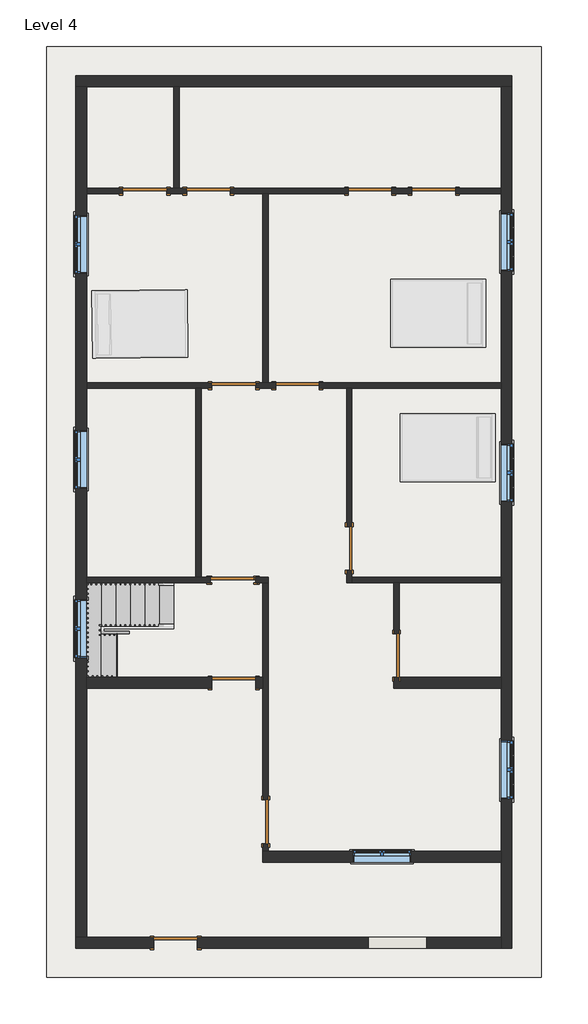
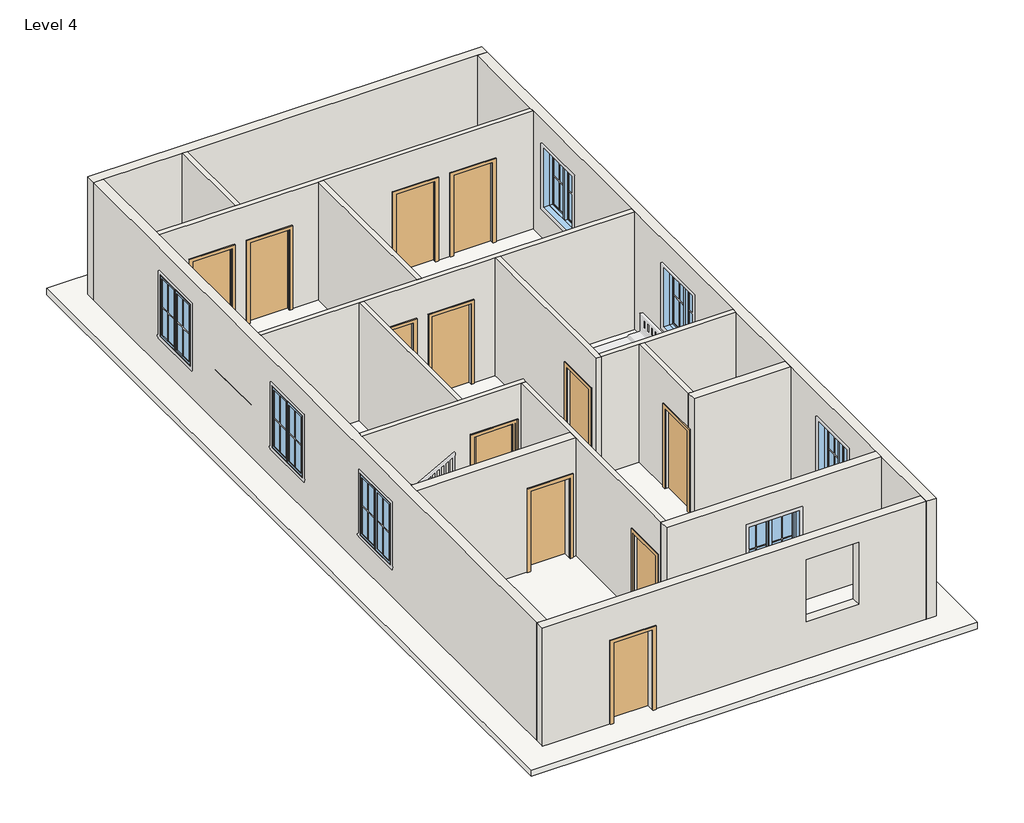
# One storey, part 1 of 2: 17 walls, 13 doors, 7 windows, 1 roof, 1 stair flight.
"""IFC4 building model written with IfcOpenShell, lengths in millimetres."""

from ifc_helpers import new_model, si_unit, frame, origin, place, context, project, spatial, polyline, outline, extrude, faceted_brep, transform, mapped, element, save
from components import door_e5f9f3c4, door_305aa2a5, door_0ca8825f, stair_flight_f33635a8, window_8377141f

model = new_model("IFC4")

# Units and contexts
model_context = context("Model", 3, world=origin())
ifc_project = project(units=[si_unit("LENGTHUNIT", "METRE", prefix="MILLI")], contexts=[model_context])

# Site, building, storey
site = spatial("IfcSite", under=ifc_project)
building = spatial("IfcBuilding", under=site)
storey = spatial("IfcBuildingStorey", under=building, Name="Level 4", Elevation=9144.0)

# Doors
placement = place(None, origin())
door_shape = door_e5f9f3c4(model_context)
element("IfcDoor", 1, ObjectType="Single-Flush : 36\" x 84\"", at=placement, inside=storey, context=model_context, shape_type="MappedRepresentation", body=[
    mapped(door_shape, transform((7442.2, 11550.65, 9144.0), x_axis=(1.0, 0.0, 0.0), y_axis=(0.0, 1.0, 0.0), z_axis=(0.0, 0.0, 1.0))),
])
element("IfcDoor", 2, ObjectType="Single-Flush : 36\" x 84\"", at=placement, inside=storey, context=model_context, shape_type="MappedRepresentation", body=[
    mapped(door_shape, transform((2717.8, 11550.65, 9144.0), x_axis=(1.0, 0.0, 0.0), y_axis=(0.0, 1.0, 0.0), z_axis=(0.0, 0.0, 1.0))),
])
element("IfcDoor", 3, ObjectType="Single-Flush : 36\" x 84\"", at=placement, inside=storey, context=model_context, shape_type="MappedRepresentation", body=[
    mapped(door_shape, transform((4584.7, 7473.95, 9144.0), x_axis=(1.0, 0.0, 0.0), y_axis=(0.0, 1.0, 0.0), z_axis=(0.0, 0.0, 1.0))),
])
element("IfcDoor", 4, ObjectType="Single-Flush : 36\" x 84\"", at=placement, inside=storey, context=model_context, shape_type="MappedRepresentation", body=[
    mapped(door_shape, transform((4546.6, 3397.25, 9144.0), x_axis=(1.0, 0.0, 0.0), y_axis=(0.0, 1.0, 0.0), z_axis=(0.0, 0.0, 1.0))),
])
element("IfcDoor", 5, ObjectType="Single-Flush : 36\" x 84\"", at=placement, inside=storey, context=model_context, shape_type="MappedRepresentation", body=[
    mapped(door_shape, transform((4584.7, 3397.25, 9144.0), x_axis=(1.0, 0.0, 0.0), y_axis=(0.0, 1.0, 0.0), z_axis=(0.0, 0.0, 1.0))),
])
element("IfcDoor", 6, ObjectType="Single-Flush : 36\" x 84\"", at=placement, inside=storey, context=model_context, shape_type="MappedRepresentation", body=[
    mapped(door_shape, transform((7004.05, 4064.0, 9144.0), x_axis=(0.0, -1.0, 0.0), y_axis=(1.0, 0.0, 0.0), z_axis=(0.0, 0.0, 1.0))),
])
element("IfcDoor", 7, ObjectType="Single-Flush : 36\" x 84\"", at=placement, inside=storey, context=model_context, shape_type="MappedRepresentation", body=[
    mapped(door_shape, transform((5251.45, -1663.7, 9144.0), x_axis=(0.0, -1.0, 0.0), y_axis=(1.0, 0.0, 0.0), z_axis=(0.0, 0.0, 1.0))),
])
door_2_shape = door_305aa2a5(model_context)
element("IfcDoor", 8, ObjectType="Single-Flush : 36\" x 84\"", at=placement, inside=storey, context=model_context, shape_type="MappedRepresentation", body=[
    mapped(door_2_shape, transform((4051.3, 11550.65, 9144.0), x_axis=(-1.0, 0.0, 0.0), y_axis=(0.0, -1.0, 0.0), z_axis=(0.0, 0.0, 1.0))),
])
element("IfcDoor", 9, ObjectType="Single-Flush : 36\" x 84\"", at=placement, inside=storey, context=model_context, shape_type="MappedRepresentation", body=[
    mapped(door_2_shape, transform((5918.2, 7473.95, 9144.0), x_axis=(-1.0, 0.0, 0.0), y_axis=(0.0, -1.0, 0.0), z_axis=(0.0, 0.0, 1.0))),
])
element("IfcDoor", 10, ObjectType="Single-Flush : 36\" x 84\"", at=placement, inside=storey, context=model_context, shape_type="MappedRepresentation", body=[
    mapped(door_2_shape, transform((7994.65, 1816.1, 9144.0), x_axis=(0.0, 1.0, 0.0), y_axis=(-1.0, 0.0, 0.0), z_axis=(0.0, 0.0, 1.0))),
])
element("IfcDoor", 11, ObjectType="Single-Flush : 36\" x 84\"", at=placement, inside=storey, context=model_context, shape_type="MappedRepresentation", body=[
    mapped(door_2_shape, transform((8775.7, 11550.65, 9144.0), x_axis=(-1.0, 0.0, 0.0), y_axis=(0.0, -1.0, 0.0), z_axis=(0.0, 0.0, 1.0))),
])
door_3_shape = door_0ca8825f(model_context)
element("IfcDoor", 12, ObjectType="Single-Flush : 36\" x 84\"", at=placement, inside=storey, context=model_context, shape_type="MappedRepresentation", body=[
    mapped(door_3_shape, transform((4584.7, 1244.6, 9144.0), x_axis=(1.0, 0.0, 0.0), y_axis=(0.0, 1.0, 0.0), z_axis=(0.0, 0.0, 1.0))),
])
element("IfcDoor", 13, ObjectType="Single-Flush : 36\" x 84\"", at=placement, inside=storey, context=model_context, shape_type="MappedRepresentation", body=[
    mapped(door_3_shape, transform((3365.5, -4203.7, 9144.0), x_axis=(1.0, 0.0, 0.0), y_axis=(0.0, 1.0, 0.0), z_axis=(0.0, 0.0, 1.0))),
])

# Roof
element("IfcRoof", 14, ObjectType="Generic - 12\"", at=placement, inside=storey, context=model_context, shape_type="SweptSolid", body=[
    extrude(outline(polyline([(660.4, 14579.6), (11023.6, 14579.6), (11023.6, -4927.6), (660.4, -4927.6), (660.4, 14579.6)])), frame((0.0, 0.0, 9144.0), z_axis=(0.0, 0.0, 1.0), x_axis=(1.0, 0.0, 0.0)), (0.0, 0.0, 1.0), 152.4),
])

# Stair flight
stair_flight_shape = stair_flight_f33635a8(model_context)
element("IfcStairFlight", 15, ObjectType="2\" Tread 1\" Nosing 1/4\" Riser", at=placement, inside=storey, context=model_context, shape_type="MappedRepresentation", body=[
    mapped(stair_flight_shape, transform((0.0, 0.0, 0.0), x_axis=(1.0, 0.0, 0.0), y_axis=(0.0, 1.0, 0.0), z_axis=(0.0, 0.0, 1.0))),
])

# Walls
element("IfcWall", 16, ObjectType="Generic - 5\"", at=placement, inside=storey, context=model_context, shape_type="SweptSolid", body=[
    extrude(outline(polyline([(3327.4, 11607.8), (3327.4, 13741.4), (3441.7, 13741.4), (3441.7, 11607.8), (3327.4, 11607.8)])), frame((0.0, 0.0, 9144.0), z_axis=(0.0, 0.0, 1.0), x_axis=(1.0, 0.0, 0.0)), (0.0, 0.0, 1.0), 3048.0),
])
element("IfcWall", 17, ObjectType="Generic - 5\"", at=placement, inside=storey, context=model_context, shape_type="Brep", body=[
    faceted_brep([(7899.4, 11493.5, 9144.0), (8318.5, 11493.5, 9144.0), (8318.5, 11493.5, 11277.6), (9232.9, 11493.5, 11277.6), (9232.9, 11493.5, 9144.0), (10185.4, 11493.5, 9144.0), (10185.4, 11493.5, 12192.0), (5308.6, 11493.5, 12192.0), (5194.3, 11493.5, 12192.0), (1498.6, 11493.5, 12192.0), (1498.6, 11493.5, 9144.0), (2260.6, 11493.5, 9144.0), (2260.6, 11493.5, 11277.6), (3175.0, 11493.5, 11277.6), (3175.0, 11493.5, 9144.0), (3594.1, 11493.5, 9144.0), (3594.1, 11493.5, 11277.6), (4508.5, 11493.5, 11277.6), (4508.5, 11493.5, 9144.0), (5194.3, 11493.5, 9144.0), (5308.6, 11493.5, 9144.0), (6985.0, 11493.5, 9144.0), (6985.0, 11493.5, 11277.6), (7899.4, 11493.5, 11277.6), (8318.5, 11607.8, 11277.6), (8318.5, 11607.8, 9144.0), (7899.4, 11607.8, 9144.0), (7899.4, 11607.8, 11277.6), (6985.0, 11607.8, 11277.6), (6985.0, 11607.8, 9144.0), (4508.5, 11607.8, 9144.0), (4508.5, 11607.8, 11277.6), (3594.1, 11607.8, 11277.6), (3594.1, 11607.8, 9144.0), (3441.7, 11607.8, 9144.0), (3327.4, 11607.8, 9144.0), (3175.0, 11607.8, 9144.0), (3175.0, 11607.8, 11277.6), (2260.6, 11607.8, 11277.6), (2260.6, 11607.8, 9144.0), (1498.6, 11607.8, 9144.0), (1498.6, 11607.8, 12192.0), (3327.4, 11607.8, 12192.0), (3441.7, 11607.8, 12192.0), (10185.4, 11607.8, 12192.0), (10185.4, 11607.8, 9144.0), (9232.9, 11607.8, 9144.0), (9232.9, 11607.8, 11277.6)], [[[0, 1, 2, 3, 4, 5, 6, 7, 8, 9, 10, 11, 12, 13, 14, 15, 16, 17, 18, 19, 20, 21, 22, 23]], [[24, 25, 26, 27, 28, 29, 30, 31, 32, 33, 34, 35, 36, 37, 38, 39, 40, 41, 42, 43, 44, 45, 46, 47]], [[11, 10, 40, 39]], [[30, 29, 21, 20, 19, 18]], [[36, 35, 34, 33, 15, 14]], [[46, 45, 5, 4]], [[26, 25, 1, 0]], [[9, 8, 7, 6, 44, 43, 42, 41]], [[6, 5, 45, 44]], [[10, 9, 41, 40]], [[27, 26, 0, 23]], [[28, 27, 23, 22]], [[29, 28, 22, 21]], [[37, 36, 14, 13]], [[38, 37, 13, 12]], [[39, 38, 12, 11]], [[16, 15, 33, 32]], [[17, 16, 32, 31]], [[18, 17, 31, 30]], [[2, 1, 25, 24]], [[3, 2, 24, 47]], [[4, 3, 47, 46]]]),
])
element("IfcWall", 18, ObjectType="Generic - 5\"", at=placement, inside=storey, context=model_context, shape_type="Brep", body=[
    faceted_brep([(5041.9, 7416.8, 11277.6), (5041.9, 7416.8, 9144.0), (5461.0, 7416.8, 9144.0), (5461.0, 7416.8, 11277.6), (6375.4, 7416.8, 11277.6), (6375.4, 7416.8, 9144.0), (6946.9, 7416.8, 9144.0), (7061.2, 7416.8, 9144.0), (10185.4, 7416.8, 9144.0), (10185.4, 7416.8, 12192.0), (7061.2, 7416.8, 12192.0), (6946.9, 7416.8, 12192.0), (3898.9, 7416.8, 12192.0), (3784.6, 7416.8, 12192.0), (1498.6, 7416.8, 12192.0), (1498.6, 7416.8, 9144.0), (3784.6, 7416.8, 9144.0), (3898.9, 7416.8, 9144.0), (4127.5, 7416.8, 9144.0), (4127.5, 7416.8, 11277.6), (5461.0, 7531.1, 9144.0), (5308.6, 7531.1, 9144.0), (5194.3, 7531.1, 9144.0), (5041.9, 7531.1, 9144.0), (5041.9, 7531.1, 11277.6), (4127.5, 7531.1, 11277.6), (4127.5, 7531.1, 9144.0), (1498.6, 7531.1, 9144.0), (1498.6, 7531.1, 12192.0), (5194.3, 7531.1, 12192.0), (5308.6, 7531.1, 12192.0), (10185.4, 7531.1, 12192.0), (10185.4, 7531.1, 9144.0), (6375.4, 7531.1, 9144.0), (6375.4, 7531.1, 11277.6), (5461.0, 7531.1, 11277.6)], [[[0, 1, 2, 3, 4, 5, 6, 7, 8, 9, 10, 11, 12, 13, 14, 15, 16, 17, 18, 19]], [[20, 21, 22, 23, 24, 25, 26, 27, 28, 29, 30, 31, 32, 33, 34, 35]], [[33, 32, 8, 7, 6, 5]], [[2, 1, 23, 22, 21, 20]], [[18, 17, 16, 15, 27, 26]], [[14, 13, 12, 11, 10, 9, 31, 30, 29, 28]], [[9, 8, 32, 31]], [[15, 14, 28, 27]], [[3, 2, 20, 35]], [[4, 3, 35, 34]], [[5, 4, 34, 33]], [[24, 23, 1, 0]], [[25, 24, 0, 19]], [[26, 25, 19, 18]]]),
])
element("IfcWall", 19, ObjectType="Generic - 5\"", at=placement, inside=storey, context=model_context, shape_type="SweptSolid", body=[
    extrude(outline(polyline([(5194.3, 7531.1), (5194.3, 11493.5), (5308.6, 11493.5), (5308.6, 7531.1), (5194.3, 7531.1)])), frame((0.0, 0.0, 9144.0), z_axis=(0.0, 0.0, 1.0), x_axis=(1.0, 0.0, 0.0)), (0.0, 0.0, 1.0), 3048.0),
])
element("IfcWall", 20, ObjectType="Generic - 5\"", at=placement, inside=storey, context=model_context, shape_type="SweptSolid", body=[
    extrude(outline(polyline([(3784.6, 3454.4), (3784.6, 7416.8), (3898.9, 7416.8), (3898.9, 3454.4), (3784.6, 3454.4)])), frame((0.0, 0.0, 9144.0), z_axis=(0.0, 0.0, 1.0), x_axis=(1.0, 0.0, 0.0)), (0.0, 0.0, 1.0), 3048.0),
])
element("IfcWall", 21, ObjectType="Generic - 5\"", at=placement, inside=storey, context=model_context, shape_type="Brep", body=[
    faceted_brep([(5308.6, 3340.1, 12192.0), (5194.3, 3340.1, 12192.0), (1498.6, 3340.1, 12192.0), (1498.6, 3340.1, 9144.0), (4089.4, 3340.1, 9144.0), (4089.4, 3340.1, 11277.6), (5041.9, 3340.1, 11277.6), (5041.9, 3340.1, 9144.0), (5194.3, 3340.1, 9144.0), (5308.6, 3340.1, 9144.0), (1498.6, 3454.4, 12192.0), (3784.6, 3454.4, 12192.0), (3898.9, 3454.4, 12192.0), (5308.6, 3454.4, 12192.0), (5308.6, 3454.4, 9144.0), (5041.9, 3454.4, 9144.0), (5041.9, 3454.4, 11277.6), (4089.4, 3454.4, 11277.6), (4089.4, 3454.4, 9144.0), (3898.9, 3454.4, 9144.0), (3784.6, 3454.4, 9144.0), (1498.6, 3454.4, 9144.0)], [[[0, 1, 2, 3, 4, 5, 6, 7, 8, 9]], [[10, 11, 12, 13, 14, 15, 16, 17, 18, 19, 20, 21]], [[3, 21, 20, 19, 18, 4]], [[14, 9, 8, 7, 15]], [[2, 1, 0, 13, 12, 11, 10]], [[3, 2, 10, 21]], [[0, 9, 14, 13]], [[5, 17, 16, 6]], [[18, 17, 5, 4]], [[6, 16, 15, 7]]]),
])
element("IfcWall", 22, ObjectType="Generic - 5\"", at=placement, inside=storey, context=model_context, shape_type="Brep", body=[
    faceted_brep([(5194.3, -2120.9, 11277.6), (5194.3, -2120.9, 9144.0), (5194.3, -2286.0, 9144.0), (5194.3, -2286.0, 12192.0), (5194.3, 1130.3, 12192.0), (5194.3, 1358.9, 12192.0), (5194.3, 3340.1, 12192.0), (5194.3, 3340.1, 9144.0), (5194.3, 1358.9, 9144.0), (5194.3, 1130.3, 9144.0), (5194.3, -1206.5, 9144.0), (5194.3, -1206.5, 11277.6), (5308.6, -2286.0, 9144.0), (5308.6, -2120.9, 9144.0), (5308.6, -2120.9, 11277.6), (5308.6, -1206.5, 11277.6), (5308.6, -1206.5, 9144.0), (5308.6, 3340.1, 9144.0), (5308.6, 3340.1, 12192.0), (5308.6, -2286.0, 12192.0)], [[[0, 1, 2, 3, 4, 5, 6, 7, 8, 9, 10, 11]], [[12, 13, 14, 15, 16, 17, 18, 19]], [[2, 1, 13, 12]], [[10, 9, 8, 7, 17, 16]], [[6, 5, 4, 3, 19, 18]], [[7, 6, 18, 17]], [[3, 2, 12, 19]], [[14, 13, 1, 0]], [[15, 14, 0, 11]], [[16, 15, 11, 10]]]),
])
element("IfcWall", 23, ObjectType="Generic - 5\"", at=placement, inside=storey, context=model_context, shape_type="Brep", body=[
    faceted_brep([(6946.9, 3606.8, 11277.6), (6946.9, 3606.8, 9144.0), (6946.9, 3340.1, 9144.0), (6946.9, 3340.1, 12192.0), (6946.9, 7416.8, 12192.0), (6946.9, 7416.8, 9144.0), (6946.9, 4521.2, 9144.0), (6946.9, 4521.2, 11277.6), (7061.2, 3340.1, 9144.0), (7061.2, 3454.4, 9144.0), (7061.2, 3606.8, 9144.0), (7061.2, 3606.8, 11277.6), (7061.2, 4521.2, 11277.6), (7061.2, 4521.2, 9144.0), (7061.2, 7416.8, 9144.0), (7061.2, 7416.8, 12192.0), (7061.2, 3454.4, 12192.0), (7061.2, 3340.1, 12192.0)], [[[0, 1, 2, 3, 4, 5, 6, 7]], [[8, 9, 10, 11, 12, 13, 14, 15, 16, 17]], [[6, 5, 14, 13]], [[2, 1, 10, 9, 8]], [[4, 3, 17, 16, 15]], [[5, 4, 15, 14]], [[3, 2, 8, 17]], [[11, 10, 1, 0]], [[12, 11, 0, 7]], [[13, 12, 7, 6]]]),
])
element("IfcWall", 24, ObjectType="Generic - 5\"", at=placement, inside=storey, context=model_context, shape_type="SweptSolid", body=[
    extrude(outline(polyline([(1358.9, 12192.0), (3340.1, 12192.0), (3340.1, 9144.0), (2273.3, 9144.0), (2273.3, 11277.6), (1358.9, 11277.6), (1358.9, 12192.0)])), frame((7937.5, 0.0, 0.0), z_axis=(1.0, 0.0, 0.0), x_axis=(0.0, 1.0, 0.0)), (0.0, 0.0, 1.0), 114.3),
])
element("IfcWall", 25, ObjectType="Generic - 5\"", at=placement, inside=storey, context=model_context, shape_type="Brep", body=[
    faceted_brep([(7061.2, 3340.1, 9144.0), (7937.5, 3340.1, 9144.0), (8051.8, 3340.1, 9144.0), (10185.4, 3340.1, 9144.0), (10185.4, 3340.1, 12192.0), (8051.8, 3340.1, 12192.0), (7937.5, 3340.1, 12192.0), (7061.2, 3340.1, 12192.0), (7061.2, 3454.4, 9144.0), (7061.2, 3454.4, 12192.0), (10185.4, 3454.4, 12192.0), (10185.4, 3454.4, 9144.0)], [[[0, 1, 2, 3, 4, 5, 6, 7]], [[8, 9, 10, 11]], [[3, 2, 1, 0, 8, 11]], [[7, 6, 5, 4, 10, 9]], [[0, 7, 9, 8]], [[4, 3, 11, 10]]]),
])
element("IfcWall", 26, ObjectType="Generic - 8\"", at=placement, inside=storey, context=model_context, shape_type="Brep", body=[
    faceted_brep([(1270.0, 13741.4, 9144.0), (1498.6, 13741.4, 9144.0), (3327.4, 13741.4, 9144.0), (3441.7, 13741.4, 9144.0), (10185.4, 13741.4, 9144.0), (10414.0, 13741.4, 9144.0), (10414.0, 13741.4, 12192.0), (10185.4, 13741.4, 12192.0), (3441.7, 13741.4, 12192.0), (3327.4, 13741.4, 12192.0), (1498.6, 13741.4, 12192.0), (1270.0, 13741.4, 12192.0), (1270.0, 13970.0, 9144.0), (1270.0, 13970.0, 12192.0), (10414.0, 13970.0, 12192.0), (10414.0, 13970.0, 9144.0)], [[[0, 1, 2, 3, 4, 5, 6, 7, 8, 9, 10, 11]], [[12, 13, 14, 15]], [[5, 4, 3, 2, 1, 0, 12, 15]], [[11, 10, 9, 8, 7, 6, 14, 13]], [[6, 5, 15, 14]], [[0, 11, 13, 12]]]),
])
element("IfcWall", 27, ObjectType="Generic - 8\"", at=placement, inside=storey, context=model_context, shape_type="Brep", body=[
    faceted_brep([(10185.4, 13741.4, 9144.0), (10185.4, 11607.8, 9144.0), (10185.4, 11493.5, 9144.0), (10185.4, 7531.1, 9144.0), (10185.4, 7416.8, 9144.0), (10185.4, 3454.4, 9144.0), (10185.4, 3340.1, 9144.0), (10185.4, 1358.9, 9144.0), (10185.4, 1130.3, 9144.0), (10185.4, -2286.0, 9144.0), (10185.4, -2514.6, 9144.0), (10185.4, -4089.4, 9144.0), (10185.4, -4318.0, 9144.0), (10185.4, -4318.0, 12192.0), (10185.4, -4089.4, 12192.0), (10185.4, -2514.6, 12192.0), (10185.4, -2286.0, 12192.0), (10185.4, 1130.3, 12192.0), (10185.4, 1358.9, 12192.0), (10185.4, 3340.1, 12192.0), (10185.4, 3454.4, 12192.0), (10185.4, 7416.8, 12192.0), (10185.4, 7531.1, 12192.0), (10185.4, 11493.5, 12192.0), (10185.4, 11607.8, 12192.0), (10185.4, 13741.4, 12192.0), (10185.4, 9874.25, 11582.4), (10185.4, 9874.25, 10058.4), (10185.4, 11093.45, 10058.4), (10185.4, 11093.45, 11582.4), (10185.4, 5035.55, 11582.4), (10185.4, 5035.55, 10058.4), (10185.4, 6254.75, 10058.4), (10185.4, 6254.75, 11582.4), (10185.4, -1187.45, 11582.4), (10185.4, -1187.45, 10058.4), (10185.4, 31.75, 10058.4), (10185.4, 31.75, 11582.4), (10414.0, 13741.4, 9144.0), (10414.0, 13741.4, 12192.0), (10414.0, -4318.0, 12192.0), (10414.0, -4318.0, 9144.0), (10414.0, 9874.25, 11582.4), (10414.0, 11093.45, 11582.4), (10414.0, 11093.45, 10058.4), (10414.0, 9874.25, 10058.4), (10414.0, 5035.55, 11582.4), (10414.0, 6254.75, 11582.4), (10414.0, 6254.75, 10058.4), (10414.0, 5035.55, 10058.4), (10414.0, -1187.45, 11582.4), (10414.0, 31.75, 11582.4), (10414.0, 31.75, 10058.4), (10414.0, -1187.45, 10058.4)], [[[0, 1, 2, 3, 4, 5, 6, 7, 8, 9, 10, 11, 12, 13, 14, 15, 16, 17, 18, 19, 20, 21, 22, 23, 24, 25], [26, 27, 28, 29], [30, 31, 32, 33], [34, 35, 36, 37]], [[38, 39, 40, 41], [42, 43, 44, 45], [46, 47, 48, 49], [50, 51, 52, 53]], [[12, 11, 10, 9, 8, 7, 6, 5, 4, 3, 2, 1, 0, 38, 41]], [[25, 24, 23, 22, 21, 20, 19, 18, 17, 16, 15, 14, 13, 40, 39]], [[0, 25, 39, 38]], [[13, 12, 41, 40]], [[27, 26, 42, 45]], [[28, 27, 45, 44]], [[29, 28, 44, 43]], [[26, 29, 43, 42]], [[31, 30, 46, 49]], [[32, 31, 49, 48]], [[33, 32, 48, 47]], [[30, 33, 47, 46]], [[35, 34, 50, 53]], [[36, 35, 53, 52]], [[37, 36, 52, 51]], [[34, 37, 51, 50]]]),
])
element("IfcWall", 28, ObjectType="Generic - 8\"", at=placement, inside=storey, context=model_context, shape_type="Brep", body=[
    faceted_brep([(10185.4, -4089.4, 9144.0), (3822.7, -4089.4, 9144.0), (3822.7, -4089.4, 11277.6), (2908.3, -4089.4, 11277.6), (2908.3, -4089.4, 9144.0), (1498.6, -4089.4, 9144.0), (1270.0, -4089.4, 9144.0), (1270.0, -4089.4, 12192.0), (1498.6, -4089.4, 12192.0), (10185.4, -4089.4, 12192.0), (7404.1, -4089.4, 11729.9484942), (7404.1, -4089.4, 10205.9484942), (8623.3, -4089.4, 10205.9484942), (8623.3, -4089.4, 11729.9484942), (3822.7, -4318.0, 11277.6), (3822.7, -4318.0, 9144.0), (10185.4, -4318.0, 9144.0), (10185.4, -4318.0, 12192.0), (1270.0, -4318.0, 12192.0), (1270.0, -4318.0, 9144.0), (2908.3, -4318.0, 9144.0), (2908.3, -4318.0, 11277.6), (7404.1, -4318.0, 11729.9484942), (8623.3, -4318.0, 11729.9484942), (8623.3, -4318.0, 10205.9484942), (7404.1, -4318.0, 10205.9484942)], [[[0, 1, 2, 3, 4, 5, 6, 7, 8, 9], [10, 11, 12, 13]], [[14, 15, 16, 17, 18, 19, 20, 21], [22, 23, 24, 25]], [[20, 19, 6, 5, 4]], [[16, 15, 1, 0]], [[9, 8, 7, 18, 17]], [[0, 9, 17, 16]], [[7, 6, 19, 18]], [[2, 1, 15, 14]], [[3, 2, 14, 21]], [[4, 3, 21, 20]], [[11, 10, 22, 25]], [[12, 11, 25, 24]], [[13, 12, 24, 23]], [[10, 13, 23, 22]]]),
])
element("IfcWall", 29, ObjectType="Generic - 8\"", at=placement, inside=storey, context=model_context, shape_type="Brep", body=[
    faceted_brep([(1498.6, -4089.4, 9144.0), (1498.6, 1130.3, 9144.0), (1498.6, 1358.9, 9144.0), (1498.6, 3340.1, 9144.0), (1498.6, 3454.4, 9144.0), (1498.6, 7416.8, 9144.0), (1498.6, 7531.1, 9144.0), (1498.6, 11493.5, 9144.0), (1498.6, 11607.8, 9144.0), (1498.6, 13741.4, 9144.0), (1498.6, 13741.4, 12192.0), (1498.6, 11607.8, 12192.0), (1498.6, 11493.5, 12192.0), (1498.6, 7531.1, 12192.0), (1498.6, 7416.8, 12192.0), (1498.6, 3454.4, 12192.0), (1498.6, 3340.1, 12192.0), (1498.6, 1358.9, 12192.0), (1498.6, 1130.3, 12192.0), (1498.6, -4089.4, 12192.0), (1498.6, 6534.15, 11582.4), (1498.6, 6534.15, 10058.4), (1498.6, 5314.95, 10058.4), (1498.6, 5314.95, 11582.4), (1498.6, 11042.65, 11582.4), (1498.6, 11042.65, 10058.4), (1498.6, 9823.45, 10058.4), (1498.6, 9823.45, 11582.4), (1498.6, 2990.85, 11582.4), (1498.6, 2990.85, 10058.4), (1498.6, 1771.65, 10058.4), (1498.6, 1771.65, 11582.4), (1270.0, -4089.4, 9144.0), (1270.0, -4089.4, 12192.0), (1270.0, 13741.4, 12192.0), (1270.0, 13741.4, 9144.0), (1270.0, 6534.15, 11582.4), (1270.0, 5314.95, 11582.4), (1270.0, 5314.95, 10058.4), (1270.0, 6534.15, 10058.4), (1270.0, 11042.65, 11582.4), (1270.0, 9823.45, 11582.4), (1270.0, 9823.45, 10058.4), (1270.0, 11042.65, 10058.4), (1270.0, 2990.85, 11582.4), (1270.0, 1771.65, 11582.4), (1270.0, 1771.65, 10058.4), (1270.0, 2990.85, 10058.4)], [[[0, 1, 2, 3, 4, 5, 6, 7, 8, 9, 10, 11, 12, 13, 14, 15, 16, 17, 18, 19], [20, 21, 22, 23], [24, 25, 26, 27], [28, 29, 30, 31]], [[32, 33, 34, 35], [36, 37, 38, 39], [40, 41, 42, 43], [44, 45, 46, 47]], [[9, 8, 7, 6, 5, 4, 3, 2, 1, 0, 32, 35]], [[19, 18, 17, 16, 15, 14, 13, 12, 11, 10, 34, 33]], [[10, 9, 35, 34]], [[0, 19, 33, 32]], [[21, 20, 36, 39]], [[22, 21, 39, 38]], [[23, 22, 38, 37]], [[20, 23, 37, 36]], [[25, 24, 40, 43]], [[26, 25, 43, 42]], [[27, 26, 42, 41]], [[24, 27, 41, 40]], [[29, 28, 44, 47]], [[30, 29, 47, 46]], [[31, 30, 46, 45]], [[28, 31, 45, 44]]]),
])
element("IfcWall", 30, ObjectType="Generic - 8\"", at=placement, inside=storey, context=model_context, shape_type="SweptSolid", body=[
    extrude(outline(polyline([(11277.6, 5041.9), (9144.0, 5041.9), (9144.0, 5194.3), (12192.0, 5194.3), (12192.0, 1498.6), (9144.0, 1498.6), (9144.0, 4127.5), (11277.6, 4127.5), (11277.6, 5041.9)])), frame((0.0, 1130.3, 0.0), z_axis=(0.0, 1.0, 0.0), x_axis=(0.0, 0.0, 1.0)), (0.0, 0.0, 1.0), 228.6),
])
element("IfcWall", 31, ObjectType="Generic - 8\"", at=placement, inside=storey, context=model_context, shape_type="Brep", body=[
    faceted_brep([(5194.3, -2514.6, 9144.0), (10185.4, -2514.6, 9144.0), (10185.4, -2514.6, 12192.0), (5194.3, -2514.6, 12192.0), (8299.45, -2514.6, 11582.4), (8299.45, -2514.6, 10058.4), (7080.25, -2514.6, 10058.4), (7080.25, -2514.6, 11582.4), (5194.3, -2286.0, 9144.0), (5194.3, -2286.0, 12192.0), (5308.6, -2286.0, 12192.0), (10185.4, -2286.0, 12192.0), (10185.4, -2286.0, 9144.0), (5308.6, -2286.0, 9144.0), (8299.45, -2286.0, 11582.4), (7080.25, -2286.0, 11582.4), (7080.25, -2286.0, 10058.4), (8299.45, -2286.0, 10058.4)], [[[0, 1, 2, 3], [4, 5, 6, 7]], [[8, 9, 10, 11, 12, 13], [14, 15, 16, 17]], [[1, 0, 8, 13, 12]], [[3, 2, 11, 10, 9]], [[0, 3, 9, 8]], [[2, 1, 12, 11]], [[5, 4, 14, 17]], [[6, 5, 17, 16]], [[7, 6, 16, 15]], [[4, 7, 15, 14]]]),
])
element("IfcWall", 32, ObjectType="Generic - 8\"", at=placement, inside=storey, context=model_context, shape_type="Brep", body=[
    faceted_brep([(7937.5, 1130.3, 9144.0), (10185.4, 1130.3, 9144.0), (10185.4, 1130.3, 12192.0), (7937.5, 1130.3, 12192.0), (7937.5, 1358.9, 9144.0), (7937.5, 1358.9, 11277.6), (7937.5, 1358.9, 12192.0), (8051.8, 1358.9, 12192.0), (10185.4, 1358.9, 12192.0), (10185.4, 1358.9, 9144.0)], [[[0, 1, 2, 3]], [[4, 5, 6, 7, 8, 9]], [[1, 0, 4, 9]], [[3, 2, 8, 7, 6]], [[0, 3, 6, 5, 4]], [[2, 1, 9, 8]]]),
])

# Windows
window_shape = window_8377141f(model_context)
element("IfcWindow", 33, ObjectType="Window-Casement-Double : 48\" x 60\"", at=placement, inside=storey, context=model_context, shape_type="MappedRepresentation", body=[
    mapped(window_shape, transform((1384.3, 5924.55, 9144.0), x_axis=(0.0, 1.0, 0.0), y_axis=(-1.0, 0.0, 0.0), z_axis=(0.0, 0.0, 1.0))),
])
element("IfcWindow", 34, ObjectType="Window-Casement-Double : 48\" x 60\"", at=placement, inside=storey, context=model_context, shape_type="MappedRepresentation", body=[
    mapped(window_shape, transform((1384.3, 10433.05, 9144.0), x_axis=(0.0, 1.0, 0.0), y_axis=(-1.0, 0.0, 0.0), z_axis=(0.0, 0.0, 1.0))),
])
element("IfcWindow", 35, ObjectType="Window-Casement-Double : 48\" x 60\"", at=placement, inside=storey, context=model_context, shape_type="MappedRepresentation", body=[
    mapped(window_shape, transform((10299.7, 10483.85, 9144.0), x_axis=(0.0, -1.0, 0.0), y_axis=(1.0, 0.0, 0.0), z_axis=(0.0, 0.0, 1.0))),
])
element("IfcWindow", 36, ObjectType="Window-Casement-Double : 48\" x 60\"", at=placement, inside=storey, context=model_context, shape_type="MappedRepresentation", body=[
    mapped(window_shape, transform((10299.7, 5645.15, 9144.0), x_axis=(0.0, -1.0, 0.0), y_axis=(1.0, 0.0, 0.0), z_axis=(0.0, 0.0, 1.0))),
])
element("IfcWindow", 37, ObjectType="Window-Casement-Double : 48\" x 60\"", at=placement, inside=storey, context=model_context, shape_type="MappedRepresentation", body=[
    mapped(window_shape, transform((10299.7, -577.85, 9144.0), x_axis=(0.0, -1.0, 0.0), y_axis=(1.0, 0.0, 0.0), z_axis=(0.0, 0.0, 1.0))),
])
element("IfcWindow", 38, ObjectType="Window-Casement-Double : 48\" x 60\"", at=placement, inside=storey, context=model_context, shape_type="MappedRepresentation", body=[
    mapped(window_shape, transform((7689.85, -2400.3, 9144.0), x_axis=(1.0, 0.0, 0.0), y_axis=(0.0, 1.0, 0.0), z_axis=(0.0, 0.0, 1.0))),
])
element("IfcWindow", 39, ObjectType="Window-Casement-Double : 48\" x 60\"", at=placement, inside=storey, context=model_context, shape_type="MappedRepresentation", body=[
    mapped(window_shape, transform((1384.3, 2381.25, 9144.0), x_axis=(0.0, 1.0, 0.0), y_axis=(-1.0, 0.0, 0.0), z_axis=(0.0, 0.0, 1.0))),
])

save(model, "model.ifc")

# Revit data of these elements
# Type "Single-Flush : 36\" x 84\""
#   Type Mark = "1"
#   Construction Type Id = "MDOOR"
#   Assembly Code = "C1020"
#   Analytic Construction = "Metal"
#   Thickness = 0' - 2"
#   Heat Transfer Coefficient (U) = 0.651978 BTU/(h·ft²·°F)
#   Height = 7' - 0"
#   Trim Projection Ext = 0' - 1"
#   Trim Projection Int = 0' - 1"
#   Trim Width = 0' - 3"
#   Width = 3' - 0"
#   Define Thermal Properties by = 1
#   Define Thermal Properties by = 1
#   Door Material = Door - Panel
#   Frame Material = Door - Frame
#   Visual Light Transmittance = 0
#   Solar Heat Gain Coefficient = 0
#   Function = (empty or 0)
#   Wall Closure = (empty or 0)
# Type "Generic - 12\""
#   Assembly Code = "B1020"
#   Layers, outside or top first: 0' - 6" no material (function 1)
# Type "Generic - 5\""
#   Assembly Code = "B2010"
#   Layers, outside or top first: 0' - 4 1/2" no material (function 1)
# Type "Generic - 8\""
#   Assembly Code = "B2010"
# Type "Window-Casement-Double : 48\" x 60\""
#   Type Mark = "17"
#   Fire Rating = "0.5h"
#   Assembly Code = "B2020100"
#   Analytic Construction = "Double glazing - domestic"
#   Frame Extension [instance default] = 0' - 0 1/4"
#   Window Inset [instance default] = 0' - 0"
#   Wall Thickness [instance default] = 0' - 6"
#   Interior Wall Closure [instance default] = 0' - 2 1/4"
#   Half Width = 2' - 0"
#   Visual Light Transmittance = 0.81
#   Thermal Resistance (R) = 1.8146 (h·ft²·°F)/BTU
#   Solar Heat Gain Coefficient = 0.76
#   Rough Width = 4' - 0 1/2"
#   Rough Height = 5' - 0 1/2"
#   Height = 5' - 0"
#   Heat Transfer Coefficient (U) = 0.5511 BTU/(h·ft²·°F)
#   Exterior Wall Closure [instance default] = 0' - 1 1/4"
#   Extension Jamb [instance default] = 0' - 2 1/4"
#   Default Sill Height = 3' - 0"
#   Width = 4' - 0"
#   Define Thermal Properties by = 0
#   Muntin Visibility = yes
#   Interior Trim Visibility [instance default] = yes
#   Exterior Trim Visibility [instance default] = yes
#   Extension Jamb Visibility [instance default] = yes
#   Interior Trim Material = Wood - Stained
#   Muntin Pattern = Muntin Pattern_2x2 : Muntin Pattern_2x2
#   Interior Trim = Trim-Window-Interior-Flat : Picture Frame
#   Interior Frame Material = Wood - Stained
#   Glass Panel Material = Glass
#   Exterior Trim Material = Clad - White
#   Exterior Trim = Trim-Window-Exterior-Flat : with Sill
#   Exterior Frame Material = Clad - White
#   Wall Closure = (empty or 0)
# Elements 1, 2, 3, 4, 5, 6, 7, 8, 9, 10, 11, 12, 13 (IfcDoor, "Single-Flush : 36\" x 84\"")
#   Phase Created = New Construction
#   Materials on its faces: "Door - Frame", "Door - Panel"
# Element 14 (IfcRoof, "Generic - 12\"")
#   built-in parameter 1001705 = 30.5 (stored number, unit not read)
#   built-in parameter 1001710 = 33615
#   Phase Created = New Construction
#   Materials on its faces: "Clad - White", "Default Roof"
# Element 15 (IfcStairFlight, "2\" Tread 1\" Nosing 1/4\" Riser")
#   Phase Created = New Construction
# Elements 16, 17, 18, 19, 20, 21, 22, 23, 24, 25 (IfcWall, "Generic - 5\"")
#   Top Offset = 0' - 0"
#   Base Offset = 0' - 0"
#   wall height = 10' - 0"
#   Phase Created = New Construction
#   Base Constraint = Level 4
#   Top Constraint = Level 5
#   Materials on its faces: "Default Wall"
# Elements 26, 27, 28, 29 (IfcWall, "Generic - 8\"")
#   Top Offset = 0' - 0"
#   Base Offset = 0' - 0"
#   Unconnected Height = 10' - 0"
#   wall height = 10' - 0"
#   Phase Created = New Construction
#   Base Constraint = Level 4
#   Materials on its faces: "Parking Stripe"
# Element 30 (IfcWall, "Generic - 8\"")
#   Top Offset = 0' - 0"
#   Base Offset = 0' - 0"
#   Unconnected Height = 10' - 0"
#   wall height = 10' - 0"
#   Phase Created = New Construction
#   Base Constraint = Level 4
# Elements 31, 32 (IfcWall, "Generic - 8\"")
#   Top Offset = 0' - 0"
#   Base Offset = 0' - 0"
#   Unconnected Height = 10' - 0"
#   wall height = 10' - 0"
#   Phase Created = New Construction
#   Base Constraint = Level 4
#   Materials on its faces: "Default Wall"
# Element 33 (IfcWindow, "Window-Casement-Double : 48\" x 60\"")
#   Mark = "22"
#   Window Inset = 0' - 0"
#   Interior Wall Closure = 0' - 2 1/4"
#   Frame Extension = 0' - 0 1/4"
#   Exterior Wall Closure = 0' - 1 1/4"
#   Interior Trim Visibility = yes
#   Exterior Trim Visibility = yes
#   Phase Created = New Construction
#   Materials on its faces: "Wood - Stained", "Glass", "Clad - White"
# Element 34 (IfcWindow, "Window-Casement-Double : 48\" x 60\"")
#   Mark = "23"
#   Window Inset = 0' - 0"
#   Interior Wall Closure = 0' - 2 1/4"
#   Frame Extension = 0' - 0 1/4"
#   Exterior Wall Closure = 0' - 1 1/4"
#   Interior Trim Visibility = yes
#   Exterior Trim Visibility = yes
#   Phase Created = New Construction
#   Materials on its faces: "Wood - Stained", "Glass", "Clad - White"
# Element 35 (IfcWindow, "Window-Casement-Double : 48\" x 60\"")
#   Mark = "24"
#   Window Inset = 0' - 0"
#   Interior Wall Closure = 0' - 2 1/4"
#   Frame Extension = 0' - 0 1/4"
#   Exterior Wall Closure = 0' - 1 1/4"
#   Interior Trim Visibility = yes
#   Exterior Trim Visibility = yes
#   Phase Created = New Construction
#   Materials on its faces: "Wood - Stained", "Glass", "Clad - White"
# Element 36 (IfcWindow, "Window-Casement-Double : 48\" x 60\"")
#   Mark = "25"
#   Window Inset = 0' - 0"
#   Interior Wall Closure = 0' - 2 1/4"
#   Frame Extension = 0' - 0 1/4"
#   Exterior Wall Closure = 0' - 1 1/4"
#   Interior Trim Visibility = yes
#   Exterior Trim Visibility = yes
#   Phase Created = New Construction
#   Materials on its faces: "Wood - Stained", "Glass", "Clad - White"
# Element 37 (IfcWindow, "Window-Casement-Double : 48\" x 60\"")
#   Mark = "26"
#   Window Inset = 0' - 0"
#   Interior Wall Closure = 0' - 2 1/4"
#   Frame Extension = 0' - 0 1/4"
#   Exterior Wall Closure = 0' - 1 1/4"
#   Interior Trim Visibility = yes
#   Exterior Trim Visibility = yes
#   Phase Created = New Construction
#   Materials on its faces: "Wood - Stained", "Glass", "Clad - White"
# Element 38 (IfcWindow, "Window-Casement-Double : 48\" x 60\"")
#   Mark = "27"
#   Window Inset = 0' - 0"
#   Interior Wall Closure = 0' - 2 1/4"
#   Frame Extension = 0' - 0 1/4"
#   Exterior Wall Closure = 0' - 1 1/4"
#   Interior Trim Visibility = yes
#   Exterior Trim Visibility = yes
#   Phase Created = New Construction
#   Materials on its faces: "Wood - Stained", "Glass", "Clad - White"
# Element 39 (IfcWindow, "Window-Casement-Double : 48\" x 60\"")
#   Mark = "28"
#   Window Inset = 0' - 0"
#   Interior Wall Closure = 0' - 2 1/4"
#   Frame Extension = 0' - 0 1/4"
#   Exterior Wall Closure = 0' - 1 1/4"
#   Interior Trim Visibility = yes
#   Exterior Trim Visibility = yes
#   Phase Created = New Construction
#   Materials on its faces: "Wood - Stained", "Glass", "Clad - White"
# Materials
#   "Door - Panel": class "Wood", colour RGB 210 159 95, transparency 0, Cost = 0
#   "Door - Frame": colour RGB 118 70 51, transparency 0, Cost = 0
#   "Wood - Stained": class "Wood", colour RGB 224 178 126, transparency 0, Cost = 0
#   "Glass": class "Glass", colour RGB 0 128 192, transparency 0.75, Description = "Soda Lime Glass", Cost = 0
#   "Clad - White": class "Wood", colour RGB 242 242 238, transparency 0, Cost = 0
#   "Default Roof": colour RGB 88 101 114, transparency 0, Cost = 0
#   "Default Wall": colour RGB 128 128 128, transparency 0, Cost = 0
#   "Parking Stripe": class "Paint", colour RGB 250 250 91, transparency 0, Cost = 0
